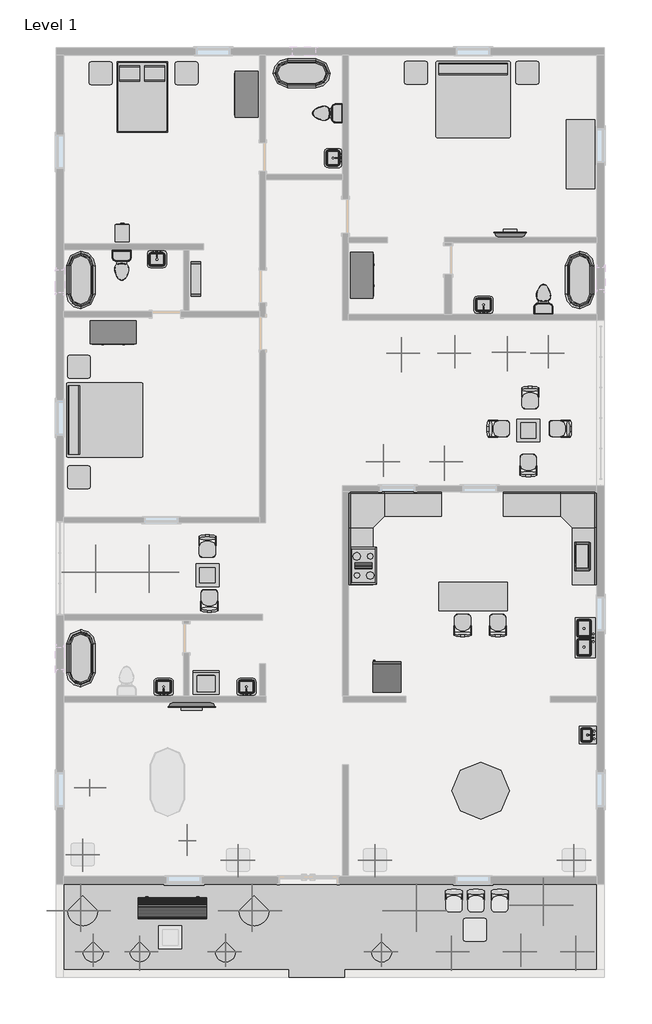
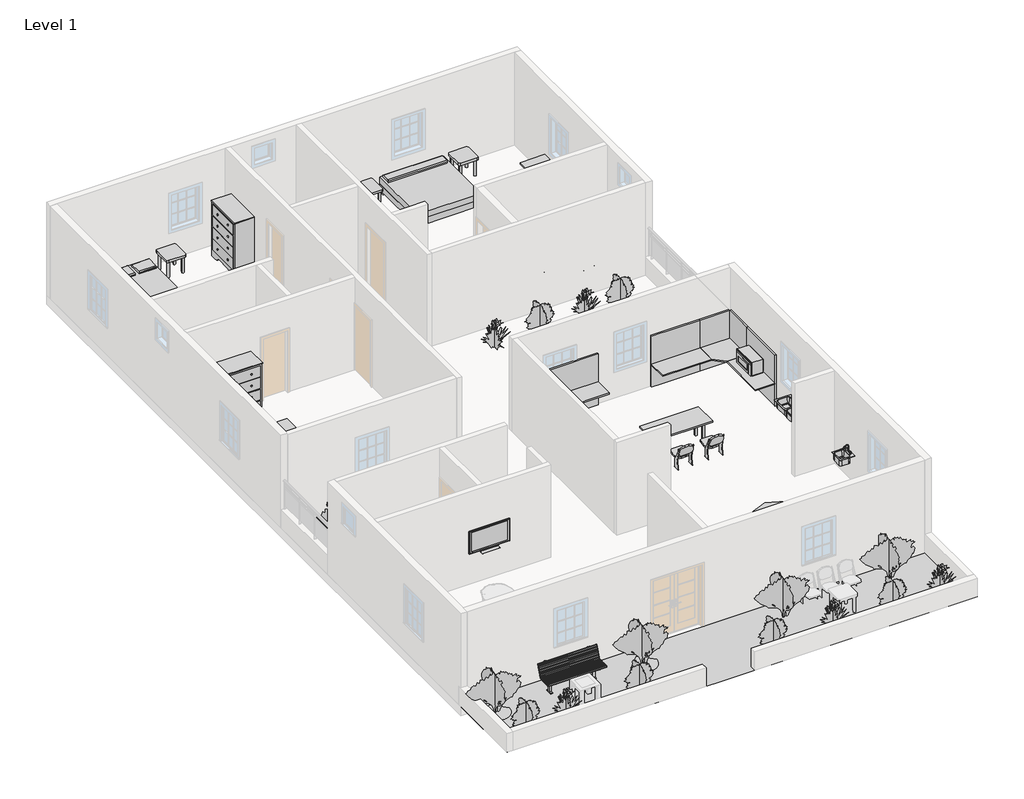
# One storey, part 3 of 3: 31 furniture elements, 24 geographic elements, 18 flow terminals, 7 proxies.
"""IFC4 building model written with IfcOpenShell, lengths in millimetres."""

from ifc_helpers import new_model, si_unit, origin, place, context, project, spatial, triangles, transform, mapped, element, save
from components import proxy_bb1e6e30, proxy_8a8d5ab2, rpc_female_69e001fa, proxy_a13a33b2, proxy_718fa39f, flow_terminal_accce45a, flow_terminal_a53be723, flow_terminal_871c2e40, flow_terminal_62a433f7, toilet_domestic_3d_toilet_domestic_3d_f7549cf7, toilet_domestic_3d_toilet_domestic_3d_183bbd19, flow_terminal_b374fae2, furniture_c8abb964, furniture_1fc5af50, furniture_552c1472, furniture_9fa109b2, furniture_3d1d9cbc, furniture_417d203a, furniture_56245f3a, furniture_fdf74506, furniture_b5c51a22, furniture_bbcc68ce, furniture_31d08a24, furniture_a5b052b6, furniture_45e3acac, geographic_element_235d1464, rpc_plant_tropical_55f6ff97, rpc_plant_tropical_6475341c, rpc_plant_tropical_agave_1_5_93a2a214, rpc_plant_tropical_jungle_flame_3_9c4808c2

model = new_model("IFC4")

# Units and contexts
model_context = context("Model", 3, world=origin())
ifc_project = project(units=[si_unit("LENGTHUNIT", "METRE", prefix="MILLI")], contexts=[model_context])

# Site, building, storey
site = spatial("IfcSite", under=ifc_project)
building = spatial("IfcBuilding", under=site)
storey = spatial("IfcBuildingStorey", under=building, Name="Level 1", Elevation=0.0)

# Proxies
placement = place(None, origin())
element("IfcBuildingElementProxy", 1, Name="Building Element Proxy", at=placement, inside=storey, context=model_context, shape_type="Tessellation", body=[
    triangles([(-15067.7442352, -9641.8998413, 0.0), (-15067.7442352, -12131.1002289, 0.0), (-437.3446349, -9641.8998413, 0.0), (-437.3446349, -12131.1002289, 0.0)], [[1, 2, 3], [4, 3, 2]], closed=False),
])
proxy_shape = proxy_bb1e6e30(model_context)
element("IfcBuildingElementProxy", 2, Name="Cook Top-4 Unit : 36\" x 20\"", ObjectType="Cook Top-4 Unit : 36\" x 20\"", at=placement, inside=storey, context=model_context, shape_type="MappedRepresentation", body=[
    mapped(proxy_shape, transform((-6863.5446525, -1158.2997829, 0.0), x_axis=(0.0, -1.0000000000000004, 0.0), y_axis=(1.0000000000000004, 0.0, 0.0), z_axis=(0.0, 0.0, 1.0))),
])
proxy_2_shape = proxy_8a8d5ab2(model_context)
element("IfcBuildingElementProxy", 3, Name="Microwave : 30\" x 16\" x 18\"", ObjectType="Microwave : 30\" x 16\" x 18\"", at=placement, inside=storey, context=model_context, shape_type="MappedRepresentation", body=[
    mapped(proxy_2_shape, transform((-668.4641467, -404.0069056, 0.0), x_axis=(0.0, -1.0000000000000007, 0.0), y_axis=(1.0000000000000007, 0.0, 0.0), z_axis=(0.0, 0.0, 1.0))),
])
rpc_female_shape = rpc_female_69e001fa(model_context)
element("IfcBuildingElementProxy", 4, Name="RPC Female", ObjectType="RPC Female", at=placement, inside=storey, context=model_context, shape_type="MappedRepresentation", body=[
    mapped(rpc_female_shape, transform((-11563.8112072, -8321.0997829, 0.0), x_axis=(-1.0000000000000004, 0.0, 0.0), y_axis=(0.0, -1.0000000000000004, 0.0), z_axis=(0.0, 0.0, 1.0))),
])
element("IfcBuildingElementProxy", 5, Name="RPC Female", ObjectType="RPC Female", at=placement, inside=storey, context=model_context, shape_type="MappedRepresentation", body=[
    mapped(rpc_female_shape, transform((-14007.2946525, -7076.4997829, 0.0), x_axis=(0.0, 1.0000000000000009, 0.0), y_axis=(-1.0000000000000009, 0.0, 0.0), z_axis=(0.0, 0.0, 1.0))),
])
proxy_3_shape = proxy_a13a33b2(model_context)
element("IfcBuildingElementProxy", 6, Name="Refrigerator : 30\" x 32\" RH", ObjectType="Refrigerator : 30\" x 32\" RH", at=placement, inside=storey, context=model_context, shape_type="MappedRepresentation", body=[
    mapped(proxy_3_shape, transform((-6246.0071525, -4137.6487544, 0.0), x_axis=(-1.0000000000000004, 0.0, 0.0), y_axis=(0.0, -1.0000000000000004, 0.0), z_axis=(0.0, 0.0, 1.0))),
])
proxy_4_shape = proxy_718fa39f(model_context)
element("IfcBuildingElementProxy", 7, Name="Washer : 27\" x 25\" x 35\"", ObjectType="Washer : 27\" x 25\" x 35\"", at=placement, inside=storey, context=model_context, shape_type="MappedRepresentation", body=[
    mapped(proxy_4_shape, transform((-11485.027184, -4545.4981611, 0.0), x_axis=(1.0000000000000009, 0.0, 0.0), y_axis=(0.0, 1.0000000000000009, 0.0), z_axis=(0.0, 0.0, 1.0))),
])

# Flow terminals
flow_terminal_shape = flow_terminal_accce45a(model_context)
element("IfcFlowTerminal", 8, ObjectType="Floor Drain - Round : 5\" Strainer - 2\" Drain", at=placement, inside=storey, context=model_context, shape_type="MappedRepresentation", body=[
    mapped(flow_terminal_shape, transform((-13924.7446525, 7020.5002171, 0.0), x_axis=(1.0, 0.0, 0.0), y_axis=(0.0, 1.0, 0.0), z_axis=(0.0, 0.0, 1.0))),
])
element("IfcFlowTerminal", 9, ObjectType="Floor Drain - Round : 5\" Strainer - 2\" Drain", at=placement, inside=storey, context=model_context, shape_type="MappedRepresentation", body=[
    mapped(flow_terminal_shape, transform((-7904.9446525, 11465.5002171, 0.0), x_axis=(1.0, 0.0, 0.0), y_axis=(0.0, 1.0, 0.0), z_axis=(0.0, 0.0, 1.0))),
])
element("IfcFlowTerminal", 10, ObjectType="Floor Drain - Round : 5\" Strainer - 2\" Drain", at=placement, inside=storey, context=model_context, shape_type="MappedRepresentation", body=[
    mapped(flow_terminal_shape, transform((-1707.3446525, 7223.7002171, 0.0), x_axis=(1.0, 0.0, 0.0), y_axis=(0.0, 1.0, 0.0), z_axis=(0.0, 0.0, 1.0))),
])
element("IfcFlowTerminal", 11, ObjectType="Floor Drain - Round : 5\" Strainer - 2\" Drain", at=placement, inside=storey, context=model_context, shape_type="MappedRepresentation", body=[
    mapped(flow_terminal_shape, transform((-10546.5446525, -4460.2997829, 0.0), x_axis=(1.0, 0.0, 0.0), y_axis=(0.0, 1.0, 0.0), z_axis=(0.0, 0.0, 1.0))),
])
flow_terminal_2_shape = flow_terminal_a53be723(model_context)
element("IfcFlowTerminal", 12, ObjectType="Sink Kitchen-Double : 42\" x 21\"", at=placement, inside=storey, context=model_context, shape_type="MappedRepresentation", body=[
    mapped(flow_terminal_2_shape, transform((-947.6900536, -3060.3105423, 0.0), x_axis=(0.0, -1.0000000000000004, 0.0), y_axis=(1.0000000000000004, 0.0, 0.0), z_axis=(0.0, 0.0, 1.0))),
])
flow_terminal_3_shape = flow_terminal_871c2e40(model_context)
element("IfcFlowTerminal", 13, ObjectType="Sink Kitchen-Island : 18\" x 18\"", at=placement, inside=storey, context=model_context, shape_type="MappedRepresentation", body=[
    mapped(flow_terminal_3_shape, transform((-884.1900536, -5651.1105423, 0.0), x_axis=(0.0, -1.0000000000000004, 0.0), y_axis=(1.0000000000000004, 0.0, 0.0), z_axis=(0.0, 0.0, 1.0))),
])
flow_terminal_4_shape = flow_terminal_62a433f7(model_context)
element("IfcFlowTerminal", 14, ObjectType="Sink Vanity-Square : 20\" x 18\"", at=placement, inside=storey, context=model_context, shape_type="MappedRepresentation", body=[
    mapped(flow_terminal_4_shape, transform((-12391.0338931, 7062.604816, 0.0), x_axis=(1.0, 0.0, 0.0), y_axis=(0.0, 1.0, 0.0), z_axis=(0.0, 0.0, 1.0))),
])
element("IfcFlowTerminal", 15, ObjectType="Sink Vanity-Square : 20\" x 18\"", at=placement, inside=storey, context=model_context, shape_type="MappedRepresentation", body=[
    mapped(flow_terminal_4_shape, transform((-7627.8900536, 9728.5894577, 0.0), x_axis=(0.0, -1.0000000000000004, 0.0), y_axis=(1.0000000000000004, 0.0, 0.0), z_axis=(0.0, 0.0, 1.0))),
])
element("IfcFlowTerminal", 16, ObjectType="Sink Vanity-Square : 20\" x 18\"", at=placement, inside=storey, context=model_context, shape_type="MappedRepresentation", body=[
    mapped(flow_terminal_4_shape, transform((-3647.4554119, 5752.8456182, 0.0), x_axis=(-0.9999999999999998, 0.0, 0.0), y_axis=(0.0, -0.9999999999999998, 0.0), z_axis=(0.0, 0.0, 1.0))),
])
element("IfcFlowTerminal", 17, ObjectType="Sink Vanity-Square : 20\" x 18\"", at=placement, inside=storey, context=model_context, shape_type="MappedRepresentation", body=[
    mapped(flow_terminal_4_shape, transform((-9972.0554119, -4432.5543818, 0.0), x_axis=(-1.0, 0.0, 0.0), y_axis=(0.0, -1.0, 0.0), z_axis=(0.0, 0.0, 1.0))),
])
element("IfcFlowTerminal", 18, ObjectType="Sink Vanity-Square : 20\" x 18\"", at=placement, inside=storey, context=model_context, shape_type="MappedRepresentation", body=[
    mapped(flow_terminal_4_shape, transform((-12181.8554119, -4432.5543818, 0.0), x_axis=(-1.0, 0.0, 0.0), y_axis=(0.0, -1.0, 0.0), z_axis=(0.0, 0.0, 1.0))),
])
toilet_domestic_3d_toilet_domestic_3d_shape = toilet_domestic_3d_toilet_domestic_3d_f7549cf7(model_context)
toilet_domestic_3d_toilet_domestic_3d_2_shape = toilet_domestic_3d_toilet_domestic_3d_183bbd19(model_context)
element("IfcFlowTerminal", 19, ObjectType="Toilet-Domestic-3D : Toilet-Domestic-3D", at=placement, inside=storey, context=model_context, shape_type="MappedRepresentation", body=[
    mapped(toilet_domestic_3d_toilet_domestic_3d_shape, transform((-13315.1446525, 6754.4041897, 0.0), x_axis=(1.0, 0.0, 0.0), y_axis=(0.0, 1.0, 0.0), z_axis=(0.0, 0.0, 1.0))),
    mapped(toilet_domestic_3d_toilet_domestic_3d_2_shape, transform((-13315.1446525, 6754.4041897, 0.0), x_axis=(1.0, 0.0, 0.0), y_axis=(0.0, 1.0, 0.0), z_axis=(0.0, 0.0, 1.0))),
])
element("IfcFlowTerminal", 20, ObjectType="Toilet-Domestic-3D : Toilet-Domestic-3D", at=placement, inside=storey, context=model_context, shape_type="MappedRepresentation", body=[
    mapped(toilet_domestic_3d_toilet_domestic_3d_shape, transform((-7917.0406798, 10906.7002171, 0.0), x_axis=(0.0, -1.0000000000000004, 0.0), y_axis=(1.0000000000000004, 0.0, 0.0), z_axis=(0.0, 0.0, 1.0))),
    mapped(toilet_domestic_3d_toilet_domestic_3d_2_shape, transform((-7917.0406798, 10906.7002171, 0.0), x_axis=(0.0, -1.0000000000000004, 0.0), y_axis=(1.0000000000000004, 0.0, 0.0), z_axis=(0.0, 0.0, 1.0))),
])
element("IfcFlowTerminal", 21, ObjectType="Toilet-Domestic-3D : Toilet-Domestic-3D", at=placement, inside=storey, context=model_context, shape_type="MappedRepresentation", body=[
    mapped(toilet_domestic_3d_toilet_domestic_3d_shape, transform((-2062.9446525, 6041.9962444, 0.0), x_axis=(-1.0, 0.0, 0.0), y_axis=(0.0, -1.0, 0.0), z_axis=(0.0, 0.0, 1.0))),
    mapped(toilet_domestic_3d_toilet_domestic_3d_2_shape, transform((-2062.9446525, 6041.9962444, 0.0), x_axis=(-1.0, 0.0, 0.0), y_axis=(0.0, -1.0, 0.0), z_axis=(0.0, 0.0, 1.0))),
])
flow_terminal_5_shape = flow_terminal_b374fae2(model_context)
element("IfcFlowTerminal", 22, ObjectType="Tub-Free Standing-3D : 30\" x 60\"", at=placement, inside=storey, context=model_context, shape_type="MappedRepresentation", body=[
    mapped(flow_terminal_5_shape, transform((-14407.3446525, 6461.7002171, 0.0), x_axis=(1.0, 0.0, 0.0), y_axis=(0.0, 1.0, 0.0), z_axis=(0.0, 0.0, 1.0))),
])
element("IfcFlowTerminal", 23, ObjectType="Tub-Free Standing-3D : 30\" x 60\"", at=placement, inside=storey, context=model_context, shape_type="MappedRepresentation", body=[
    mapped(flow_terminal_5_shape, transform((-8514.5446525, 11973.5002171, 0.0), x_axis=(0.0, 1.0000000000000002, 0.0), y_axis=(-1.0000000000000002, 0.0, 0.0), z_axis=(0.0, 0.0, 1.0))),
])
element("IfcFlowTerminal", 24, ObjectType="Tub-Free Standing-3D : 30\" x 60\"", at=placement, inside=storey, context=model_context, shape_type="MappedRepresentation", body=[
    mapped(flow_terminal_5_shape, transform((-1097.7446525, 6461.7002171, 0.0), x_axis=(1.0, 0.0, 0.0), y_axis=(0.0, 1.0, 0.0), z_axis=(0.0, 0.0, 1.0))),
])
element("IfcFlowTerminal", 25, ObjectType="Tub-Free Standing-3D : 30\" x 60\"", at=placement, inside=storey, context=model_context, shape_type="MappedRepresentation", body=[
    mapped(flow_terminal_5_shape, transform((-14407.3446525, -3622.0997829, 0.0), x_axis=(1.0, 0.0, 0.0), y_axis=(0.0, 1.0, 0.0), z_axis=(0.0, 0.0, 1.0))),
])

# Furniture
furniture_shape = furniture_c8abb964(model_context)
element("IfcFurniture", 26, ObjectType="Bed-Box : Double 53\" x 74\"", at=placement, inside=storey, context=model_context, shape_type="MappedRepresentation", body=[
    mapped(furniture_shape, transform((-13108.1971115, 11572.9297253, 0.0), x_axis=(1.0, 0.0, 0.0), y_axis=(0.0, 1.0, 0.0), z_axis=(0.0, 0.0, 1.0))),
])
furniture_2_shape = furniture_1fc5af50(model_context)
element("IfcFurniture", 27, ObjectType="Bed-Standard.0001 : King 78\" x 80\"", at=placement, inside=storey, context=model_context, shape_type="MappedRepresentation", body=[
    mapped(furniture_2_shape, transform((-4214.0331771, 11320.5952991, 0.0), x_axis=(1.0, 0.0, 0.0), y_axis=(0.0, 1.0, 0.0), z_axis=(0.0, 0.0, 1.0))),
])
element("IfcFurniture", 28, ObjectType="Bed-Standard.0001 : King 78\" x 80\"", at=placement, inside=storey, context=model_context, shape_type="MappedRepresentation", body=[
    mapped(furniture_2_shape, transform((-13817.9397345, 2456.4116925, 0.0), x_axis=(0.0, 1.0000000000000002, 0.0), y_axis=(-1.0000000000000002, 0.0, 0.0), z_axis=(0.0, 0.0, 1.0))),
])
furniture_3_shape = furniture_552c1472(model_context)
element("IfcFurniture", 29, ObjectType="Cabinet-File 3 Drawer : 15\" x 18\"", at=placement, inside=storey, context=model_context, shape_type="MappedRepresentation", body=[
    mapped(furniture_3_shape, transform((-13430.3410995, 7564.165917, 0.0), x_axis=(-1.0, 0.0, 0.0), y_axis=(0.0, -1.0, 0.0), z_axis=(0.0, 0.0, 1.0))),
])
furniture_4_shape = furniture_9fa109b2(model_context)
element("IfcFurniture", 30, ObjectType="Dresser : 48\" x 72\" x 24\"", at=placement, inside=storey, context=model_context, shape_type="MappedRepresentation", body=[
    mapped(furniture_4_shape, transform((-9624.5816984, 11145.5069573, 0.0), x_axis=(0.0, -1.0000000000000004, 0.0), y_axis=(1.0000000000000004, 0.0, 0.0), z_axis=(0.0, 0.0, 1.0))),
])
element("IfcFurniture", 31, ObjectType="Dresser : 48\" x 72\" x 24\"", at=placement, inside=storey, context=model_context, shape_type="MappedRepresentation", body=[
    mapped(furniture_4_shape, transform((-7277.5076066, 6857.8934769, 0.0), x_axis=(0.0, 1.0000000000000002, 0.0), y_axis=(-1.0000000000000002, 0.0, 0.0), z_axis=(0.0, 0.0, 1.0))),
])
element("IfcFurniture", 32, ObjectType="Dresser : 48\" x 72\" x 24\"", at=placement, inside=storey, context=model_context, shape_type="MappedRepresentation", body=[
    mapped(furniture_4_shape, transform((-13274.5513926, 5427.8631712, 0.0), x_axis=(1.0, 0.0, 0.0), y_axis=(0.0, 1.0, 0.0), z_axis=(0.0, 0.0, 1.0))),
])
furniture_5_shape = furniture_3d1d9cbc(model_context)
element("IfcFurniture", 33, ObjectType="Seating-Auditorium : 18\" x 24\" x 30\"", at=placement, inside=storey, context=model_context, shape_type="MappedRepresentation", body=[
    mapped(furniture_5_shape, transform((-4382.6725213, -2948.3751927, 0.0), x_axis=(1.0000000000000007, 0.0, 0.0), y_axis=(0.0, 1.0000000000000007, 0.0), z_axis=(0.0, 0.0, 1.0))),
])
element("IfcFurniture", 34, ObjectType="Seating-Auditorium : 18\" x 24\" x 30\"", at=placement, inside=storey, context=model_context, shape_type="MappedRepresentation", body=[
    mapped(furniture_5_shape, transform((-3442.8725213, -2948.3751927, 0.0), x_axis=(1.0, 0.0, 0.0), y_axis=(0.0, 1.0, 0.0), z_axis=(0.0, 0.0, 1.0))),
])
element("IfcFurniture", 35, ObjectType="Seating-Auditorium : 18\" x 24\" x 30\"", at=placement, inside=storey, context=model_context, shape_type="MappedRepresentation", body=[
    mapped(furniture_5_shape, transform((-10868.4167836, -435.0243731, 0.0), x_axis=(-1.000000000000001, 0.0, 0.0), y_axis=(0.0, -1.000000000000001, 0.0), z_axis=(0.0, 0.0, 1.0))),
])
element("IfcFurniture", 36, ObjectType="Seating-Auditorium : 18\" x 24\" x 30\"", at=placement, inside=storey, context=model_context, shape_type="MappedRepresentation", body=[
    mapped(furniture_5_shape, transform((-11139.0725213, -2287.9751927, 0.0), x_axis=(1.0000000000000002, 0.0, 0.0), y_axis=(0.0, 1.0000000000000002, 0.0), z_axis=(0.0, 0.0, 1.0))),
])
element("IfcFurniture", 37, ObjectType="Seating-Auditorium : 18\" x 24\" x 30\"", at=placement, inside=storey, context=model_context, shape_type="MappedRepresentation", body=[
    mapped(furniture_5_shape, transform((-2257.8167836, 3527.3756269, 0.0), x_axis=(-1.0000000000000004, 0.0, 0.0), y_axis=(0.0, -1.0000000000000004, 0.0), z_axis=(0.0, 0.0, 1.0))),
])
element("IfcFurniture", 38, ObjectType="Seating-Auditorium : 18\" x 24\" x 30\"", at=placement, inside=storey, context=model_context, shape_type="MappedRepresentation", body=[
    mapped(furniture_5_shape, transform((-2630.0725213, 1318.8248073, 0.0), x_axis=(1.0000000000000009, 0.0, 0.0), y_axis=(0.0, 1.0000000000000009, 0.0), z_axis=(0.0, 0.0, 1.0))),
])
element("IfcFurniture", 39, ObjectType="Seating-Auditorium : 18\" x 24\" x 30\"", at=placement, inside=storey, context=model_context, shape_type="MappedRepresentation", body=[
    mapped(furniture_5_shape, transform((-1415.8692426, 2338.5723482, 0.0), x_axis=(0.0, 1.000000000000001, 0.0), y_axis=(-1.000000000000001, 0.0, 0.0), z_axis=(0.0, 0.0, 1.0))),
])
element("IfcFurniture", 40, ObjectType="Seating-Auditorium : 18\" x 24\" x 30\"", at=placement, inside=storey, context=model_context, shape_type="MappedRepresentation", body=[
    mapped(furniture_5_shape, transform((-3472.0200623, 2660.0280859, 0.0), x_axis=(0.0, -1.0000000000000002, 0.0), y_axis=(1.0000000000000002, 0.0, 0.0), z_axis=(0.0, 0.0, 1.0))),
])
furniture_6_shape = furniture_417d203a(model_context)
element("IfcFurniture", 41, ObjectType="Shelving : 36\" x 10\" x 72\"", at=placement, inside=storey, context=model_context, shape_type="MappedRepresentation", body=[
    mapped(furniture_6_shape, transform((-11638.7446525, 6487.1002171, 0.0), x_axis=(0.0, 1.0000000000000002, 0.0), y_axis=(-1.0000000000000002, 0.0, 0.0), z_axis=(0.0, 0.0, 1.0))),
])
furniture_7_shape = furniture_56245f3a(model_context)
element("IfcFurniture", 42, ObjectType="TV - Flat Screen : 32\"", at=placement, inside=storey, context=model_context, shape_type="MappedRepresentation", body=[
    mapped(furniture_7_shape, transform((-2955.8891666, 7665.8124392, 914.4), x_axis=(-1.0000000000000004, 0.0, 0.0), y_axis=(0.0, -1.0000000000000004, 0.0), z_axis=(0.0, 0.0, 1.0))),
])
furniture_8_shape = furniture_fdf74506(model_context)
element("IfcFurniture", 43, ObjectType="TV - Flat Screen : 50\"", at=placement, inside=storey, context=model_context, shape_type="MappedRepresentation", body=[
    mapped(furniture_8_shape, transform((-11444.3001383, -4863.2111705, 1041.4), x_axis=(1.0, 0.0, 0.0), y_axis=(0.0, 1.0, 0.0), z_axis=(0.0, 0.0, 1.0))),
])
furniture_9_shape = furniture_b5c51a22(model_context)
element("IfcFurniture", 44, ObjectType="Table-Coffee : 24\" x 24\" x 24\"", at=placement, inside=storey, context=model_context, shape_type="MappedRepresentation", body=[
    mapped(furniture_9_shape, transform((-11047.4104192, -1507.5108607, 0.0), x_axis=(1.0, 0.0, 0.0), y_axis=(0.0, 1.0, 0.0), z_axis=(0.0, 0.0, 1.0))),
])
element("IfcFurniture", 45, ObjectType="Table-Coffee : 24\" x 24\" x 24\"", at=placement, inside=storey, context=model_context, shape_type="MappedRepresentation", body=[
    mapped(furniture_9_shape, transform((-2487.6104192, 2353.2891393, 0.0), x_axis=(1.0, 0.0, 0.0), y_axis=(0.0, 1.0, 0.0), z_axis=(0.0, 0.0, 1.0))),
])
furniture_10_shape = furniture_bbcc68ce(model_context)
element("IfcFurniture", 46, ObjectType="Table-Dining Round w Chairs : 60\" Diameter", at=placement, inside=storey, context=model_context, shape_type="MappedRepresentation", body=[
    mapped(furniture_10_shape, transform((-3843.0266197, -6967.8210944, 0.0), x_axis=(1.0, 0.0, 0.0), y_axis=(0.0, 1.0, 0.0), z_axis=(0.0, 0.0, 1.0))),
])
furniture_11_shape = furniture_31d08a24(model_context)
element("IfcFurniture", 47, ObjectType="Table-End : 24\" x 24\"", at=placement, inside=storey, context=model_context, shape_type="MappedRepresentation", body=[
    mapped(furniture_11_shape, transform((-14182.4782828, 11821.1002171, 0.0), x_axis=(1.0, 0.0, 0.0), y_axis=(0.0, 1.0, 0.0), z_axis=(0.0, 0.0, 1.0))),
])
element("IfcFurniture", 48, ObjectType="Table-End : 24\" x 24\"", at=placement, inside=storey, context=model_context, shape_type="MappedRepresentation", body=[
    mapped(furniture_11_shape, transform((-11896.4782828, 11821.1002171, 0.0), x_axis=(1.0, 0.0, 0.0), y_axis=(0.0, 1.0, 0.0), z_axis=(0.0, 0.0, 1.0))),
])
element("IfcFurniture", 49, ObjectType="Table-End : 24\" x 24\"", at=placement, inside=storey, context=model_context, shape_type="MappedRepresentation", body=[
    mapped(furniture_11_shape, transform((-2803.2782828, 11833.8002171, 0.0), x_axis=(1.0, 0.0, 0.0), y_axis=(0.0, 1.0, 0.0), z_axis=(0.0, 0.0, 1.0))),
])
element("IfcFurniture", 50, ObjectType="Table-End : 24\" x 24\"", at=placement, inside=storey, context=model_context, shape_type="MappedRepresentation", body=[
    mapped(furniture_11_shape, transform((-5775.0782828, 11833.8002171, 0.0), x_axis=(1.0, 0.0, 0.0), y_axis=(0.0, 1.0, 0.0), z_axis=(0.0, 0.0, 1.0))),
])
element("IfcFurniture", 51, ObjectType="Table-End : 24\" x 24\"", at=placement, inside=storey, context=model_context, shape_type="MappedRepresentation", body=[
    mapped(furniture_11_shape, transform((-14766.6782828, 3997.9002171, 0.0), x_axis=(1.0, 0.0, 0.0), y_axis=(0.0, 1.0, 0.0), z_axis=(0.0, 0.0, 1.0))),
])
element("IfcFurniture", 52, ObjectType="Table-End : 24\" x 24\"", at=placement, inside=storey, context=model_context, shape_type="MappedRepresentation", body=[
    mapped(furniture_11_shape, transform((-14766.6782828, 1051.5002171, 0.0), x_axis=(1.0, 0.0, 0.0), y_axis=(0.0, 1.0, 0.0), z_axis=(0.0, 0.0, 1.0))),
])
furniture_12_shape = furniture_a5b052b6(model_context)
element("IfcFurniture", 53, ObjectType="Table-Rectangular : 72\" x 30\"", at=placement, inside=storey, context=model_context, shape_type="MappedRepresentation", body=[
    mapped(furniture_12_shape, transform((-1072.3446525, 9814.5002171, 0.0), x_axis=(0.0, 1.0000000000000002, 0.0), y_axis=(-1.0000000000000002, 0.0, 0.0), z_axis=(0.0, 0.0, 1.0))),
])
element("IfcFurniture", 54, ObjectType="Table-Rectangular : 72\" x 30\"", at=placement, inside=storey, context=model_context, shape_type="MappedRepresentation", body=[
    mapped(furniture_12_shape, transform((-3942.5446525, -1971.0997829, 0.0), x_axis=(1.0, 0.0, 0.0), y_axis=(0.0, 1.0, 0.0), z_axis=(0.0, 0.0, 1.0))),
])
furniture_13_shape = furniture_45e3acac(model_context)
element("IfcFurniture", 55, ObjectType="Work Station Cubicle : 96\" x 96\"", at=placement, inside=storey, context=model_context, shape_type="MappedRepresentation", body=[
    mapped(furniture_13_shape, transform((-145.5216449, 691.1684649, 0.0), x_axis=(0.0, -1.0000000000000004, 0.0), y_axis=(1.0000000000000004, 0.0, 0.0), z_axis=(0.0, 0.0, 1.0))),
])
element("IfcFurniture", 56, ObjectType="Work Station Cubicle : 96\" x 96\"", at=placement, inside=storey, context=model_context, shape_type="MappedRepresentation", body=[
    mapped(furniture_13_shape, transform((-7138.2129003, 1317.9232247, 0.0), x_axis=(1.0, 0.0, 0.0), y_axis=(0.0, 1.0, 0.0), z_axis=(0.0, 0.0, 1.0))),
])

# Geographic elements
geographic_element_shape = geographic_element_235d1464(model_context)
element("IfcGeographicElement", 57, ObjectType="Park Bench : 72\"", at=placement, inside=storey, context=model_context, shape_type="MappedRepresentation", body=[
    mapped(geographic_element_shape, transform((-11968.9446525, -10251.4997829, 0.0), x_axis=(1.0, 0.0, 0.0), y_axis=(0.0, 1.0, 0.0), z_axis=(0.0, 0.0, 1.0))),
])
rpc_plant_tropical_shape = rpc_plant_tropical_55f6ff97(model_context)
element("IfcGeographicElement", 58, ObjectType="RPC Plant - Tropical", at=placement, inside=storey, context=model_context, shape_type="MappedRepresentation", body=[
    mapped(rpc_plant_tropical_shape, transform((-5847.5446525, 4505.9002171, 0.0), x_axis=(1.0, 0.0, 0.0), y_axis=(0.0, 1.0, 0.0), z_axis=(0.0, 0.0, 1.0))),
])
element("IfcGeographicElement", 59, ObjectType="RPC Plant - Tropical", at=placement, inside=storey, context=model_context, shape_type="MappedRepresentation", body=[
    mapped(rpc_plant_tropical_shape, transform((-4704.5446525, 1610.3002171, 0.0), x_axis=(1.0, 0.0, 0.0), y_axis=(0.0, 1.0, 0.0), z_axis=(0.0, 0.0, 1.0))),
])
element("IfcGeographicElement", 60, ObjectType="RPC Plant - Tropical", at=placement, inside=storey, context=model_context, shape_type="MappedRepresentation", body=[
    mapped(rpc_plant_tropical_shape, transform((-3028.1446525, 4531.3002171, 0.0), x_axis=(1.0, 0.0, 0.0), y_axis=(0.0, 1.0, 0.0), z_axis=(0.0, 0.0, 1.0))),
])
element("IfcGeographicElement", 61, ObjectType="RPC Plant - Tropical", at=placement, inside=storey, context=model_context, shape_type="MappedRepresentation", body=[
    mapped(rpc_plant_tropical_shape, transform((-1199.3446525, -11445.2997829, 0.0), x_axis=(1.0, 0.0, 0.0), y_axis=(0.0, 1.0, 0.0), z_axis=(0.0, 0.0, 1.0))),
])
element("IfcGeographicElement", 62, ObjectType="RPC Plant - Tropical", at=placement, inside=storey, context=model_context, shape_type="MappedRepresentation", body=[
    mapped(rpc_plant_tropical_shape, transform((-4526.7446525, -11445.2997829, 0.0), x_axis=(1.0, 0.0, 0.0), y_axis=(0.0, 1.0, 0.0), z_axis=(0.0, 0.0, 1.0))),
])
element("IfcGeographicElement", 63, ObjectType="RPC Plant - Tropical", at=placement, inside=storey, context=model_context, shape_type="MappedRepresentation", body=[
    mapped(rpc_plant_tropical_shape, transform((-12832.5446525, -11445.2997829, 0.0), x_axis=(1.0, 0.0, 0.0), y_axis=(0.0, 1.0, 0.0), z_axis=(0.0, 0.0, 1.0))),
])
rpc_plant_tropical_2_shape = rpc_plant_tropical_6475341c(model_context)
element("IfcGeographicElement", 64, ObjectType="RPC Plant - Tropical", at=placement, inside=storey, context=model_context, shape_type="MappedRepresentation", body=[
    mapped(rpc_plant_tropical_2_shape, transform((-13950.1446525, -1323.3997829, 0.0), x_axis=(1.0, 0.0, 0.0), y_axis=(0.0, 1.0, 0.0), z_axis=(0.0, 0.0, 1.0))),
])
element("IfcGeographicElement", 65, ObjectType="RPC Plant - Tropical", at=placement, inside=storey, context=model_context, shape_type="MappedRepresentation", body=[
    mapped(rpc_plant_tropical_2_shape, transform((-12527.7446525, -1323.3997829, 0.0), x_axis=(1.0, 0.0, 0.0), y_axis=(0.0, 1.0, 0.0), z_axis=(0.0, 0.0, 1.0))),
])
element("IfcGeographicElement", 66, ObjectType="RPC Plant - Tropical", at=placement, inside=storey, context=model_context, shape_type="MappedRepresentation", body=[
    mapped(rpc_plant_tropical_2_shape, transform((-14356.5446525, -10353.0997829, 0.0), x_axis=(1.0, 0.0, 0.0), y_axis=(0.0, 1.0, 0.0), z_axis=(0.0, 0.0, 1.0))),
])
element("IfcGeographicElement", 67, ObjectType="RPC Plant - Tropical", at=placement, inside=storey, context=model_context, shape_type="MappedRepresentation", body=[
    mapped(rpc_plant_tropical_2_shape, transform((-9784.5446525, -10353.0997829, 0.0), x_axis=(1.0, 0.0, 0.0), y_axis=(0.0, 1.0, 0.0), z_axis=(0.0, 0.0, 1.0))),
])
element("IfcGeographicElement", 68, ObjectType="RPC Plant - Tropical", at=placement, inside=storey, context=model_context, shape_type="MappedRepresentation", body=[
    mapped(rpc_plant_tropical_2_shape, transform((-5390.3446525, -10353.0997829, 0.0), x_axis=(1.0, 0.0, 0.0), y_axis=(0.0, 1.0, 0.0), z_axis=(0.0, 0.0, 1.0))),
])
element("IfcGeographicElement", 69, ObjectType="RPC Plant - Tropical", at=placement, inside=storey, context=model_context, shape_type="MappedRepresentation", body=[
    mapped(rpc_plant_tropical_2_shape, transform((-2012.1446525, -10200.6997829, 0.0), x_axis=(1.0, 0.0, 0.0), y_axis=(0.0, 1.0, 0.0), z_axis=(0.0, 0.0, 1.0))),
])
rpc_plant_tropical_agave_1_5_shape = rpc_plant_tropical_agave_1_5_93a2a214(model_context)
element("IfcGeographicElement", 70, ObjectType="RPC Plant - Tropical : Agave - 1.5'", at=placement, inside=storey, context=model_context, shape_type="MappedRepresentation", body=[
    mapped(rpc_plant_tropical_agave_1_5_shape, transform((-14356.5446525, -8854.4997829, 609.6), x_axis=(1.0, 0.0, 0.0), y_axis=(0.0, 1.0, 0.0), z_axis=(0.0, 0.0, 1.0))),
])
element("IfcGeographicElement", 71, ObjectType="RPC Plant - Tropical : Agave - 1.5'", at=placement, inside=storey, context=model_context, shape_type="MappedRepresentation", body=[
    mapped(rpc_plant_tropical_agave_1_5_shape, transform((-10216.3446525, -9000.5497829, 609.6), x_axis=(1.0, 0.0, 0.0), y_axis=(0.0, 1.0, 0.0), z_axis=(0.0, 0.0, 1.0))),
])
element("IfcGeographicElement", 72, ObjectType="RPC Plant - Tropical : Agave - 1.5'", at=placement, inside=storey, context=model_context, shape_type="MappedRepresentation", body=[
    mapped(rpc_plant_tropical_agave_1_5_shape, transform((-6558.7446525, -9000.5497829, 609.6), x_axis=(1.0, 0.0, 0.0), y_axis=(0.0, 1.0, 0.0), z_axis=(0.0, 0.0, 1.0))),
])
element("IfcGeographicElement", 73, ObjectType="RPC Plant - Tropical : Agave - 1.5'", at=placement, inside=storey, context=model_context, shape_type="MappedRepresentation", body=[
    mapped(rpc_plant_tropical_agave_1_5_shape, transform((-1250.1446525, -9000.5497829, 609.6), x_axis=(1.0, 0.0, 0.0), y_axis=(0.0, 1.0, 0.0), z_axis=(0.0, 0.0, 1.0))),
])
rpc_plant_tropical_jungle_flame_3_shape = rpc_plant_tropical_jungle_flame_3_9c4808c2(model_context)
element("IfcGeographicElement", 74, ObjectType="RPC Plant - Tropical : Jungle Flame - 3'", at=placement, inside=storey, context=model_context, shape_type="MappedRepresentation", body=[
    mapped(rpc_plant_tropical_jungle_flame_3_shape, transform((-1935.9446525, 4505.9002171, 0.0), x_axis=(1.0, 0.0, 0.0), y_axis=(0.0, 1.0, 0.0), z_axis=(0.0, 0.0, 1.0))),
])
element("IfcGeographicElement", 75, ObjectType="RPC Plant - Tropical : Jungle Flame - 3'", at=placement, inside=storey, context=model_context, shape_type="MappedRepresentation", body=[
    mapped(rpc_plant_tropical_jungle_flame_3_shape, transform((-4425.1446525, 4505.9002171, 0.0), x_axis=(1.0, 0.0, 0.0), y_axis=(0.0, 1.0, 0.0), z_axis=(0.0, 0.0, 1.0))),
])
element("IfcGeographicElement", 76, ObjectType="RPC Plant - Tropical : Jungle Flame - 3'", at=placement, inside=storey, context=model_context, shape_type="MappedRepresentation", body=[
    mapped(rpc_plant_tropical_jungle_flame_3_shape, transform((-6330.1446525, 1610.3002171, 0.0), x_axis=(1.0, 0.0, 0.0), y_axis=(0.0, 1.0, 0.0), z_axis=(0.0, 0.0, 1.0))),
])
element("IfcGeographicElement", 77, ObjectType="RPC Plant - Tropical : Jungle Flame - 3'", at=placement, inside=storey, context=model_context, shape_type="MappedRepresentation", body=[
    mapped(rpc_plant_tropical_jungle_flame_3_shape, transform((-14077.1446525, -11445.2997829, 0.0), x_axis=(1.0, 0.0, 0.0), y_axis=(0.0, 1.0, 0.0), z_axis=(0.0, 0.0, 1.0))),
])
element("IfcGeographicElement", 78, ObjectType="RPC Plant - Tropical : Jungle Flame - 3'", at=placement, inside=storey, context=model_context, shape_type="MappedRepresentation", body=[
    mapped(rpc_plant_tropical_jungle_flame_3_shape, transform((-10546.5446525, -11445.2997829, 0.0), x_axis=(1.0, 0.0, 0.0), y_axis=(0.0, 1.0, 0.0), z_axis=(0.0, 0.0, 1.0))),
])
element("IfcGeographicElement", 79, ObjectType="RPC Plant - Tropical : Jungle Flame - 3'", at=placement, inside=storey, context=model_context, shape_type="MappedRepresentation", body=[
    mapped(rpc_plant_tropical_jungle_flame_3_shape, transform((-6380.9446525, -11445.2997829, 0.0), x_axis=(1.0, 0.0, 0.0), y_axis=(0.0, 1.0, 0.0), z_axis=(0.0, 0.0, 1.0))),
])
element("IfcGeographicElement", 80, ObjectType="RPC Plant - Tropical : Jungle Flame - 3'", at=placement, inside=storey, context=model_context, shape_type="MappedRepresentation", body=[
    mapped(rpc_plant_tropical_jungle_flame_3_shape, transform((-2672.5446525, -11445.2997829, 0.0), x_axis=(1.0, 0.0, 0.0), y_axis=(0.0, 1.0, 0.0), z_axis=(0.0, 0.0, 1.0))),
])

save(model, "model.ifc")

# Revit data of these elements
# Type "Cook Top-4 Unit : 36\" x 20\""
#   Assembly Code = "E1090400"
#   Depth = 2' - 0"
#   Width = 3' - 0"
#   Burner Material = Steel, Chrome Plated
#   Cooktop Material = Steel, Polished
#   Default Elevation = 0
# Type "Microwave : 30\" x 16\" x 18\""
#   Assembly Code = "E1090400"
#   Depth = 1' - 4"
#   Height = 1' - 6"
#   Width = 2' - 6"
#   Microwave Material = Laminate, Ivory, Matte
#   Default Elevation = 0
# Type "RPC Female"
#   built-in parameter 1005195 = "RPC-8-FXA2-QQQ0-UGV2-6"
#   Height = 0
# Type "Refrigerator : 30\" x 32\" RH"
#   Label = "REF."
#   Assembly Code = "E1090400"
#   Depth = 2' - 7 3/4"
#   Handle = 2' - 3"
#   Height = 5' - 10"
#   Rear Clearance = 0' - 2"
#   Top Door Height = 1' - 8"
#   Width = 2' - 5 3/8"
#   Material = Steel, Paint Finish, Ivory, Glossy
#   Default Elevation = 0
# Type "Washer : 27\" x 25\" x 35\""
#   Label = "W"
#   Assembly Code = "E1090400"
#   Depth = 2' - 1"
#   Height = 2' - 11"
#   Width = 2' - 3"
#   Washer Material = Steel, Paint Finish, Ivory, Matte
#   Default Elevation = 0
# Type "Floor Drain - Round : 5\" Strainer - 2\" Drain"
#   WFU = 2
#   Strainer Height = 0' - 3 1/4"
#   Strainer Radius = 0' - 2 1/2"
#   Strainer Diameter = 0' - 5"
#   Radius 6 = 0' - 0 5/8"
#   Radius 5 = 0' - 1 1/4"
#   Radius 4 = 0' - 1 7/8"
#   Radius 2 = 0' - 3.04167"
#   Radius 1 = 0' - 2.02083"
#   Radius 3 = 0' - 2 1/32"
#   Pipe Radius = 1"
#   Pipe Diameter = 2"
#   Height 2 = 0' - 0.725"
#   Height 1 = 0' - 1 13/16"
#   Body Radius = 0' - 4 1/16"
#   Body Height = 0' - 3 5/8"
#   Body Diameter = 0' - 8 1/8"
#   Drain Material = none
#   HWFU = 0
#   Default Elevation = 0
#   CWFU = 0
# Type "Sink Kitchen-Double : 42\" x 21\""
#   Assembly Code = "D2010410"
#   Counter Height = 3' - 0"
#   Depth = 1' - 9"
#   Width = 3' - 6"
#   Faucet Material = Steel, Polished
#   Sink Material = Steel, Polished
#   Default Elevation = 0
# Type "Sink Kitchen-Island : 18\" x 18\""
#   Assembly Code = "D2010410"
#   Counter Height = 3' - 0"
#   Depth = 1' - 6"
#   Width = 1' - 6"
#   Faucet Material = Steel, Polished
#   Sink Material = Steel, Polished
#   Default Elevation = 0
# Type "Sink Vanity-Square : 20\" x 18\""
#   Assembly Code = "D2010400"
#   Counter Height = 2' - 7"
#   Depth = 1' - 6"
#   Width = 1' - 8"
#   Basin Material = Porcelain, Linen
#   Faucet Material = Steel, Polished
#   Default Elevation = 0
# Type "Toilet-Domestic-3D : Toilet-Domestic-3D"
#   Assembly Code = "D2010110"
#   Toilet - Bowl/Basin Material = Porcelain, Linen
#   Toilet - Seat Material = Laminate, Linen, Matte
#   Default Elevation = 0
# Type "Tub-Free Standing-3D : 30\" x 60\""
#   Assembly Code = "D2010110"
#   Height = 1' - 6"
#   Length = 5' - 0"
#   Width = 2' - 6"
#   Tub Material = Porcelain, Ivory
#   Default Elevation = 0
# Type "Bed-Box : Double 53\" x 74\""
#   Assembly Code = "E2020200"
#   Length = 6' - 2"
#   Width = 4' - 5"
#   Frame Material = Birch
#   Mattress Material = Linen, White
#   Default Elevation = 0
# Type "Bed-Standard.0001 : King 78\" x 80\""
#   Assembly Code = "E2020200"
#   Length = 6' - 8"
#   Width = 6' - 6"
#   Leg Material = Steel, Chrome Plated
#   Mattress Material = Linen, White
#   Default Elevation = 0
# Type "Cabinet-File 3 Drawer : 15\" x 18\""
#   Assembly Code = "E2020200"
#   Depth = 1' - 6"
#   Height = 3' - 5"
#   Width = 1' - 3"
#   Cabinet Material = Steel, Paint Finish, Ivory, Glossy
#   Handle Material = Steel, Chrome Plated
#   Default Elevation = 0
# Type "Dresser : 48\" x 72\" x 24\""
#   Assembly Code = "E2020200"
#   Depth = 2' - 0"
#   Height = 6' - 0"
#   Width = 4' - 0"
#   Dresser Material = Laminate - Ivory, Glossy
#   Drawer Material = Laminate, Ivory, Matte
#   Knob Material = Cherry
#   Default Elevation = 0
# Type "Seating-Auditorium : 18\" x 24\" x 30\""
#   Assembly Code = "E2020200"
#   Seat Material = Linen, Beige
#   Frame Material = Steel, Paint Finish, Dark Gray, Matte
#   Default Elevation = 0
# Type "Shelving : 36\" x 10\" x 72\""
#   Assembly Code = "E2020200"
#   Depth = 0' - 10"
#   Height = 6' - 0"
#   Width = 3' - 0"
#   Shelving Unit Material = Birch
#   Default Elevation = 0
# Type "TV - Flat Screen : 32\""
#   SinAng = 0' - 0.0193"
#   L = 2' - 3.79372"
#   H = 1' - 3.6354"
#   Thickness = 0' - 4.33071"
#   Diagonal = 2' - 7.88976"
#   CosAng = 0' - 0.03431"
#   Stand [instance default] = yes
#   Default Elevation = 0
# Type "TV - Flat Screen : 50\""
#   SinAng = 0' - 0.0193"
#   L = 3' - 7.57782"
#   H = 2' - 0.51477"
#   Thickness = 0' - 4.33071"
#   Diagonal = 4' - 2"
#   CosAng = 0' - 0.03431"
#   Stand [instance default] = yes
#   Default Elevation = 0
# Type "Table-Coffee : 24\" x 24\" x 24\""
#   Assembly Code = "E2020200"
#   Height = 2' - 0"
#   Length = 2' - 0"
#   Width = 2' - 0"
#   Top Material = none
#   Frame Material = none
#   Default Elevation = 0
# Type "Table-Dining Round w Chairs : 60\" Diameter"
#   Assembly Code = "E2020200"
#   Radius = 2' - 6"
#   Diameter = 5' - 0"
#   Height = 2' - 6"
#   Chairs = 6
#   Base Material = Pine
#   Top Material = Laminate, Linen, Matte
#   Default Elevation = 0
# Type "Table-End : 24\" x 24\""
#   Assembly Code = "E2020200"
#   Height = 2' - 0"
#   Length = 2' - 0"
#   Width = 2' - 0"
#   Base Material = Birch
#   Top Material = Laminate, Ivory, Matte
#   Default Elevation = 0
# Type "Table-Rectangular : 72\" x 30\""
#   Assembly Code = "E2020200"
#   Height = 2' - 6"
#   Length = 6' - 0"
#   Width = 2' - 6"
#   Base Material = Birch
#   Top Material = Birch
#   Default Elevation = 0
# Type "Work Station Cubicle : 96\" x 96\""
#   Assembly Code = "E2020"
#   Desktop Height = 2' - 6"
#   Desktop1 Width = 2' - 0"
#   Desktop2 Width = 2' - 0"
#   Panel Height = 5' - 6"
#   Panel1 Length = 5' - 0"
#   Panel2 Length = 5' - 0"
#   Cube Panel Material = Textile - Light Gray
#   Work Top Material = Laminate, Ivory, Matte
#   Default Elevation = 0
# Type "Park Bench : 72\""
#   Length = 6' - 0"
#   Seat Material = Wood - Teak
#   Frame Material = Steel, Paint Finish, Dark Gray, Matte
# Type "RPC Plant - Tropical"
#   built-in parameter 1005198 = "{2, 15},{39, RPC-16-FWM5-GM7X-C67P-4000-ST1L-LVER-AU},{1, 0},{1, 0},{2, 13},{1, 8},{5, Color},{1, 0},{1, 0},{3, 0.8},{3, 0.8},{3, 0.8},{1, 8},{7, BBoxMin},{1, 0},{1, 0},{1, 0},{1, 0},{1, 0},{1, 8},{7, BBoxMax},{1, 0},{1, 0},{1, 0},{1, 0},{1, 0},{2, 11},{9, RPCTypeId},{1, 0},{1, 0},{39, RPC-16-FWM5-GM7X-C67P-4000-ST1L-LVER-AU},{1, 6},{14, RPCPlantHeight},{1, 0},{1, 0},{1, 3},{2, 11},{7, keyword},{1, 0},{1, 0},{35, :RPCs:Shrubs [General]:Geometry:RPC},{2, 11},{8, category},{1, 0},{1, 0},{16, Shrubs [General]},{2, 11},{12, LocalizedUID},{1, 0},{1, 0},{10, Crane Lily},{2, 14},{6, Height},{1, 0},{1, 0},{1, 3},{1, 2},{16, Cast Reflections},{1, 0},{1, 0},{1, 0},{1, 2},{12, Cast Shadows},{1, 0},{1, 0},{1, 1},{1, 2},{9, Lock View},{1, 0},{1, 0},{1, 0},{1, 4},{5, ViewC},{1, 0},{1, 0},{1, 0},{21, assetlibrary_base.fbx},{1, 5},"
#   built-in parameter 1005195 = "RPC-16-FWM5-GM7X-C67P-4000-ST1L-LVER-AU"
#   Assembly Code = "G2050500"
#   Height = 3' - 0"
#   Default Elevation = 0
# Type "RPC Plant - Tropical"
#   built-in parameter 1005198 = "{2, 15},{39, RPC-16-G3GK-N2Q0-PN0G-6000-ST1L-LVER-AU},{1, 0},{1, 0},{2, 13},{1, 8},{5, Color},{1, 0},{1, 0},{3, 0.8},{3, 0.8},{3, 0.8},{1, 8},{7, BBoxMin},{1, 0},{1, 0},{1, 0},{1, 0},{1, 0},{1, 8},{7, BBoxMax},{1, 0},{1, 0},{1, 0},{1, 0},{1, 0},{2, 11},{9, RPCTypeId},{1, 0},{1, 0},{39, RPC-16-G3GK-N2Q0-PN0G-6000-ST1L-LVER-AU},{1, 6},{14, RPCPlantHeight},{1, 0},{1, 0},{3, 4.5},{2, 11},{7, keyword},{1, 0},{1, 0},{35, :RPCs:Shrubs [General]:Geometry:RPC},{2, 11},{8, category},{1, 0},{1, 0},{16, Shrubs [General]},{2, 11},{12, LocalizedUID},{1, 0},{1, 0},{12, Honey Myrtle},{2, 14},{6, Height},{1, 0},{1, 0},{3, 4.5},{1, 2},{16, Cast Reflections},{1, 0},{1, 0},{1, 0},{1, 2},{12, Cast Shadows},{1, 0},{1, 0},{1, 1},{1, 2},{9, Lock View},{1, 0},{1, 0},{1, 0},{1, 4},{5, ViewC},{1, 0},{1, 0},{1, 0},{21, assetlibrary_base.fbx},{1, 5},"
#   built-in parameter 1005195 = "RPC-16-G3GK-N2Q0-PN0G-6000-ST1L-LVER-AU"
#   Assembly Code = "G2050500"
#   Height = 4' - 6"
#   Default Elevation = 0
# Type "RPC Plant - Tropical : Agave - 1.5'"
#   built-in parameter 1005198 = "{2, 15},{39, RPC-16-G1GJ-63FX-7K5P-N000-ST1L-LVER-AU},{1, 0},{1, 0},{2, 13},{1, 8},{5, Color},{1, 0},{1, 0},{3, 0.8},{3, 0.8},{3, 0.8},{1, 8},{7, BBoxMin},{1, 0},{1, 0},{1, 0},{1, 0},{1, 0},{1, 8},{7, BBoxMax},{1, 0},{1, 0},{1, 0},{1, 0},{1, 0},{2, 11},{9, RPCTypeId},{1, 0},{1, 0},{39, RPC-16-G1GJ-63FX-7K5P-N000-ST1L-LVER-AU},{1, 6},{14, RPCPlantHeight},{1, 0},{1, 0},{3, 1.5},{2, 11},{7, keyword},{1, 0},{1, 0},{35, :RPCs:Plants [General]:Geometry:RPC},{2, 11},{8, category},{1, 0},{1, 0},{16, Plants [General]},{2, 11},{12, LocalizedUID},{1, 0},{1, 0},{5, Agave},{2, 14},{6, Height},{1, 0},{1, 0},{3, 1.5},{1, 2},{16, Cast Reflections},{1, 0},{1, 0},{1, 0},{1, 2},{12, Cast Shadows},{1, 0},{1, 0},{1, 1},{1, 2},{9, Lock View},{1, 0},{1, 0},{1, 0},{1, 4},{5, ViewC},{1, 0},{1, 0},{1, 0},{21, assetlibrary_base.fbx},{1, 5},"
#   built-in parameter 1005195 = "RPC-16-G1GJ-63FX-7K5P-N000-ST1L-LVER-AU"
#   Type Comments = "Agave"
#   Assembly Code = "G2050500"
#   Height = 1' - 6"
#   Default Elevation = 0
# Type "RPC Plant - Tropical : Jungle Flame - 3'"
#   built-in parameter 1005198 = "{2, 15},{39, RPC-16-FUVJ-JWG0-MWGK-8000-ST1L-LVER-AU},{1, 0},{1, 0},{2, 13},{1, 8},{5, Color},{1, 0},{1, 0},{3, 0.8},{3, 0.8},{3, 0.8},{1, 8},{7, BBoxMin},{1, 0},{1, 0},{1, 0},{1, 0},{1, 0},{1, 8},{7, BBoxMax},{1, 0},{1, 0},{1, 0},{1, 0},{1, 0},{2, 11},{9, RPCTypeId},{1, 0},{1, 0},{39, RPC-16-FUVJ-JWG0-MWGK-8000-ST1L-LVER-AU},{1, 6},{14, RPCPlantHeight},{1, 0},{1, 0},{1, 3},{2, 11},{7, keyword},{1, 0},{1, 0},{35, :RPCs:Shrubs [General]:Geometry:RPC},{2, 11},{8, category},{1, 0},{1, 0},{16, Shrubs [General]},{2, 11},{12, LocalizedUID},{1, 0},{1, 0},{12, Jungle Flame},{2, 14},{6, Height},{1, 0},{1, 0},{1, 3},{1, 2},{16, Cast Reflections},{1, 0},{1, 0},{1, 0},{1, 2},{12, Cast Shadows},{1, 0},{1, 0},{1, 1},{1, 2},{9, Lock View},{1, 0},{1, 0},{1, 0},{1, 4},{5, ViewC},{1, 0},{1, 0},{1, 0},{21, assetlibrary_base.fbx},{1, 5},"
#   built-in parameter 1005195 = "RPC-16-FUVJ-JWG0-MWGK-8000-ST1L-LVER-AU"
#   Type Comments = "Jungle Flame"
#   Assembly Code = "G2050500"
#   Height = 3' - 0"
#   Default Elevation = 0
# Element 1 (IfcBuildingElementProxy)
#   Material = none
#   Phase Created = New Construction
# Element 2 (IfcBuildingElementProxy, "Cook Top-4 Unit : 36\" x 20\"")
#   Phase Created = New Construction
#   Materials on its faces: "Steel, Chrome Plated", "Steel, Polished"
# Element 3 (IfcBuildingElementProxy, "Microwave : 30\" x 16\" x 18\"")
#   Phase Created = New Construction
#   Materials on its faces: "Laminate, Ivory, Matte", "Glass"
# Elements 4, 5 (IfcBuildingElementProxy, "RPC Female")
#   Phase Created = New Construction
# Element 6 (IfcBuildingElementProxy, "Refrigerator : 30\" x 32\" RH")
#   Phase Created = New Construction
#   Materials on its faces: "Steel, Paint Finish, Ivory, Glossy", "Steel, Chrome Plated"
# Element 7 (IfcBuildingElementProxy, "Washer : 27\" x 25\" x 35\"")
#   Phase Created = New Construction
#   Materials on its faces: "Steel, Paint Finish, Ivory, Matte"
# Element 8 (IfcFlowTerminal, "Floor Drain - Round : 5\" Strainer - 2\" Drain")
#   Mark = "4"
#   Phase Created = New Construction
# Element 9 (IfcFlowTerminal, "Floor Drain - Round : 5\" Strainer - 2\" Drain")
#   Mark = "8"
#   Phase Created = New Construction
# Element 10 (IfcFlowTerminal, "Floor Drain - Round : 5\" Strainer - 2\" Drain")
#   Mark = "13"
#   Phase Created = New Construction
# Element 11 (IfcFlowTerminal, "Floor Drain - Round : 5\" Strainer - 2\" Drain")
#   Mark = "21"
#   Phase Created = New Construction
# Element 12 (IfcFlowTerminal, "Sink Kitchen-Double : 42\" x 21\"")
#   Mark = "20"
#   Phase Created = New Construction
#   Materials on its faces: "Steel, Polished"
# Element 13 (IfcFlowTerminal, "Sink Kitchen-Island : 18\" x 18\"")
#   Mark = "19"
#   Phase Created = New Construction
#   Materials on its faces: "Steel, Polished"
# Element 14 (IfcFlowTerminal, "Sink Vanity-Square : 20\" x 18\"")
#   Mark = "3"
#   Phase Created = New Construction
#   Materials on its faces: "Porcelain, Linen", "Steel, Polished"
# Element 15 (IfcFlowTerminal, "Sink Vanity-Square : 20\" x 18\"")
#   Mark = "7"
#   Phase Created = New Construction
#   Materials on its faces: "Porcelain, Linen", "Steel, Polished"
# Element 16 (IfcFlowTerminal, "Sink Vanity-Square : 20\" x 18\"")
#   Mark = "12"
#   Phase Created = New Construction
#   Materials on its faces: "Porcelain, Linen", "Steel, Polished"
# Element 17 (IfcFlowTerminal, "Sink Vanity-Square : 20\" x 18\"")
#   Mark = "15"
#   Phase Created = New Construction
#   Materials on its faces: "Porcelain, Linen", "Steel, Polished"
# Element 18 (IfcFlowTerminal, "Sink Vanity-Square : 20\" x 18\"")
#   Mark = "16"
#   Phase Created = New Construction
#   Materials on its faces: "Porcelain, Linen", "Steel, Polished"
# Element 19 (IfcFlowTerminal, "Toilet-Domestic-3D : Toilet-Domestic-3D")
#   Mark = "2"
#   Phase Created = New Construction
#   Materials on its faces: "Porcelain, Linen", "Laminate, Linen, Matte"
# Element 20 (IfcFlowTerminal, "Toilet-Domestic-3D : Toilet-Domestic-3D")
#   Mark = "6"
#   Phase Created = New Construction
#   Materials on its faces: "Porcelain, Linen", "Laminate, Linen, Matte"
# Element 21 (IfcFlowTerminal, "Toilet-Domestic-3D : Toilet-Domestic-3D")
#   Mark = "11"
#   Phase Created = New Construction
#   Materials on its faces: "Porcelain, Linen", "Laminate, Linen, Matte"
# Element 22 (IfcFlowTerminal, "Tub-Free Standing-3D : 30\" x 60\"")
#   Mark = "1"
#   Phase Created = New Construction
#   Materials on its faces: "Porcelain, Ivory"
# Element 23 (IfcFlowTerminal, "Tub-Free Standing-3D : 30\" x 60\"")
#   Mark = "5"
#   Phase Created = New Construction
#   Materials on its faces: "Porcelain, Ivory"
# Element 24 (IfcFlowTerminal, "Tub-Free Standing-3D : 30\" x 60\"")
#   Mark = "9"
#   Phase Created = New Construction
#   Materials on its faces: "Porcelain, Ivory"
# Element 25 (IfcFlowTerminal, "Tub-Free Standing-3D : 30\" x 60\"")
#   Mark = "14"
#   Phase Created = New Construction
#   Materials on its faces: "Porcelain, Ivory"
# Element 26 (IfcFurniture, "Bed-Box : Double 53\" x 74\"")
#   Phase Created = New Construction
#   Materials on its faces: "Birch", "Linen, White"
# Elements 27, 28 (IfcFurniture, "Bed-Standard.0001 : King 78\" x 80\"")
#   Phase Created = New Construction
#   Materials on its faces: "Linen, White", "Steel, Chrome Plated"
# Element 29 (IfcFurniture, "Cabinet-File 3 Drawer : 15\" x 18\"")
#   Phase Created = New Construction
#   Materials on its faces: "Steel, Chrome Plated", "Steel, Paint Finish, Ivory, Glossy"
# Elements 30, 31, 32 (IfcFurniture, "Dresser : 48\" x 72\" x 24\"")
#   Phase Created = New Construction
#   Materials on its faces: "Laminate, Ivory, Matte", "Cherry", "Laminate - Ivory, Glossy"
# Elements 33, 34, 35, 36, 37, 38, 39, 40 (IfcFurniture, "Seating-Auditorium : 18\" x 24\" x 30\"")
#   Phase Created = New Construction
#   Materials on its faces: "Steel, Paint Finish, Dark Gray, Matte", "Linen, Beige"
# Element 41 (IfcFurniture, "Shelving : 36\" x 10\" x 72\"")
#   Phase Created = New Construction
#   Materials on its faces: "Birch"
# Element 42 (IfcFurniture, "TV - Flat Screen : 32\"")
#   Stand = yes
#   Phase Created = New Construction
#   Materials on its faces: "TV - Black", "TV - Glass", "TV - Screen"
# Element 43 (IfcFurniture, "TV - Flat Screen : 50\"")
#   Stand = yes
#   Phase Created = New Construction
#   Materials on its faces: "TV - Black", "TV - Glass", "TV - Screen"
# Elements 44, 45 (IfcFurniture, "Table-Coffee : 24\" x 24\" x 24\"")
#   Phase Created = New Construction
#   Materials on its faces: "Glass - Clear, Grey"
# Element 46 (IfcFurniture, "Table-Dining Round w Chairs : 60\" Diameter")
#   Phase Created = New Construction
#   Materials on its faces: "Pine", "Laminate, Linen, Matte"
# Elements 47, 48, 49, 50, 51, 52 (IfcFurniture, "Table-End : 24\" x 24\"")
#   Phase Created = New Construction
#   Materials on its faces: "Laminate, Ivory, Matte", "Birch"
# Elements 53, 54 (IfcFurniture, "Table-Rectangular : 72\" x 30\"")
#   Phase Created = New Construction
#   Materials on its faces: "Birch"
# Elements 55, 56 (IfcFurniture, "Work Station Cubicle : 96\" x 96\"")
#   Phase Created = New Construction
#   Materials on its faces: "Textile - Light Gray", "Laminate, Ivory, Matte"
# Element 57 (IfcGeographicElement, "Park Bench : 72\"")
#   Phase Created = New Construction
#   Materials on its faces: "Wood - Teak", "Steel, Paint Finish, Dark Gray, Matte"
# Elements 58, 59, 60, 61, 62, 63, 64, 65, 66, 67, 68, 69 (IfcGeographicElement, "RPC Plant - Tropical")
#   Phase Created = New Construction
# Elements 70, 71, 72, 73 (IfcGeographicElement, "RPC Plant - Tropical : Agave - 1.5'")
#   Phase Created = New Construction
# Elements 74, 75, 76, 77, 78, 79, 80 (IfcGeographicElement, "RPC Plant - Tropical : Jungle Flame - 3'")
#   Phase Created = New Construction
# Materials
#   "Steel, Chrome Plated": class "Metal", colour RGB 17 17 17, transparency 0, Description = "Chromiuim plated steel", Cost = 0
#   "Steel, Polished": class "Metal", colour RGB 57 57 57, transparency 0, Description = "Polished steel", Cost = 0
#   "Laminate, Ivory, Matte": class "Plastic", colour RGB 247 247 239, transparency 0, Description = "Plastic Laminate - Ivory, Matte", Cost = 0
#   "Steel, Paint Finish, Ivory, Glossy": class "Metal", colour RGB 247 247 239, transparency 0, Description = "Steel, paint finish, ivory, glossy", Cost = 0
#   "Steel, Paint Finish, Ivory, Matte": class "Metal", colour RGB 247 247 239, transparency 0, Description = "Steel, paint finish, ivory, matte", Cost = 0
#   "Porcelain, Linen": class "Ceramic", colour RGB 249 239 230, transparency 0, Description = "Porcelain, linen", Cost = 0
#   "Laminate, Linen, Matte": class "Plastic", colour RGB 249 239 230, transparency 0, Description = "Plastic Laminate - Linen, Matte", Cost = 0
#   "Porcelain, Ivory": class "Ceramic", colour RGB 247 247 239, transparency 0, Description = "Porcelain, ivory", Cost = 0
#   "Birch": class "Wood", colour RGB 224 178 126, transparency 0, Description = "Betula Alleghaniensis", Cost = 0
#   "Linen, White": class "Textile", colour RGB 247 247 239, transparency 0, Description = "Linen, white", Cost = 0
#   "Laminate - Ivory, Glossy": colour RGB 247 247 239, transparency 0
#   "Cherry": class "Wood", colour RGB 226 177 128, transparency 0, Description = "Prunus Serotina", Cost = 0
#   "Linen, Beige": class "Textile", colour RGB 249 239 230, transparency 0, Description = "Linen, beige", Cost = 0
#   "Steel, Paint Finish, Dark Gray, Matte": class "Metal", colour RGB 0 0 0, transparency 0, Description = "Steel, paint finish, dark gray, matte", Cost = 0
#   "Pine": class "Wood", colour RGB 223 192 134, transparency 0, Description = "Pinus Echinata", Cost = 0
#   "Textile - Light Gray": class "Fabric", colour RGB 204 204 204, transparency 0
#   "Wood - Teak": class "Wood", colour RGB 145 112 90, transparency 0
#   "Glass": class "Glass", colour RGB 0 128 192, transparency 0.75, Description = "Soda Lime Glass", Cost = 0
#   "TV - Black": colour RGB 49 49 49, transparency 0
#   "TV - Glass": colour RGB 157 157 157, transparency 0.9
#   "TV - Screen": colour RGB 0 0 0, transparency 0
#   "Glass - Clear, Grey": class "Glass", colour RGB 252 255 255, transparency 0.64
